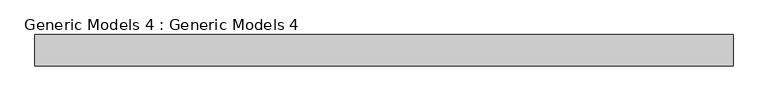
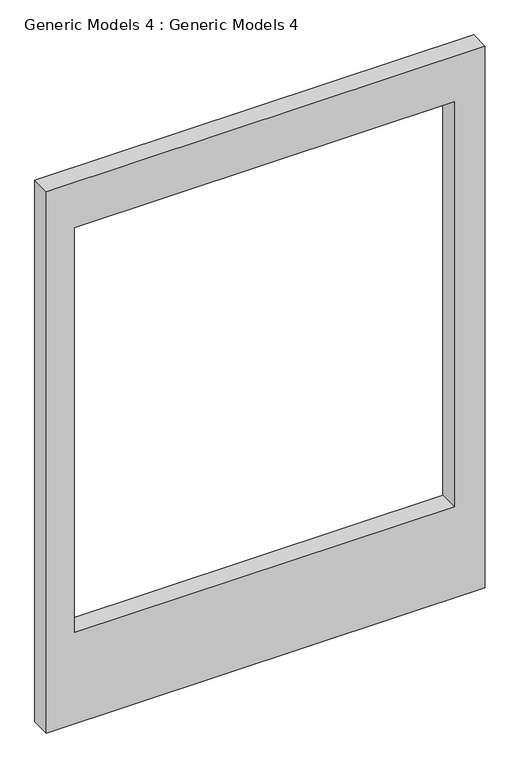
"""IFC4 building model written with IfcOpenShell, lengths in millimetres: proxy geometry, Generic Models 4 : Generic Models 4."""

from ifc_helpers import new_model, si_unit, frame, origin, place, context, project, spatial, polyline, outline, extrude, source, transform, mapped, element, save


def generic_models_4_generic_models_4_8888209d(model_context):
    return source(origin(), model_context, "Body", "SweptSolid", [
        extrude(outline(polyline([(3265.5319917, -16727.530247), (3265.5319917, -18988.130247), (319.1319917, -18988.130247), (319.1319917, -16727.530247), (3265.5319917, -16727.530247)]), holes=[polyline([(3018.6850236, -16885.429089), (815.9706649, -16885.429089), (815.9706649, -18841.229089), (3018.6850236, -18841.229089), (3018.6850236, -16885.429089)])]), frame((0.0, -2974.6468048, 0.0), z_axis=(0.0, 1.0, 0.0), x_axis=(0.0, 0.0, 1.0)), (0.0, 0.0, 1.0), 101.6),
    ])


if __name__ == "__main__":
    model = new_model("IFC4")
    model_context = context("Model", 3, world=origin())
    ifc_project = project(units=[si_unit("LENGTHUNIT", "METRE", prefix="MILLI")], contexts=[model_context])
    site = spatial("IfcSite", under=ifc_project)
    building = spatial("IfcBuilding", under=site)
    placement = place(None, origin())
    generic_models_4_generic_models_4_shape = generic_models_4_generic_models_4_8888209d(model_context)
    element("IfcBuildingElementProxy", 1, Name="Generic Models 4 : Generic Models 4", ObjectType="Generic Models 4 : Generic Models 4", at=placement, inside=building, context=model_context, shape_type="MappedRepresentation", body=[
        mapped(generic_models_4_generic_models_4_shape, transform((0.0, 0.0, 0.0), x_axis=(1.0, 0.0, 0.0), y_axis=(0.0, 1.0, 0.0), z_axis=(0.0, 0.0, 1.0))),
    ])
    save(model, "model.ifc")
